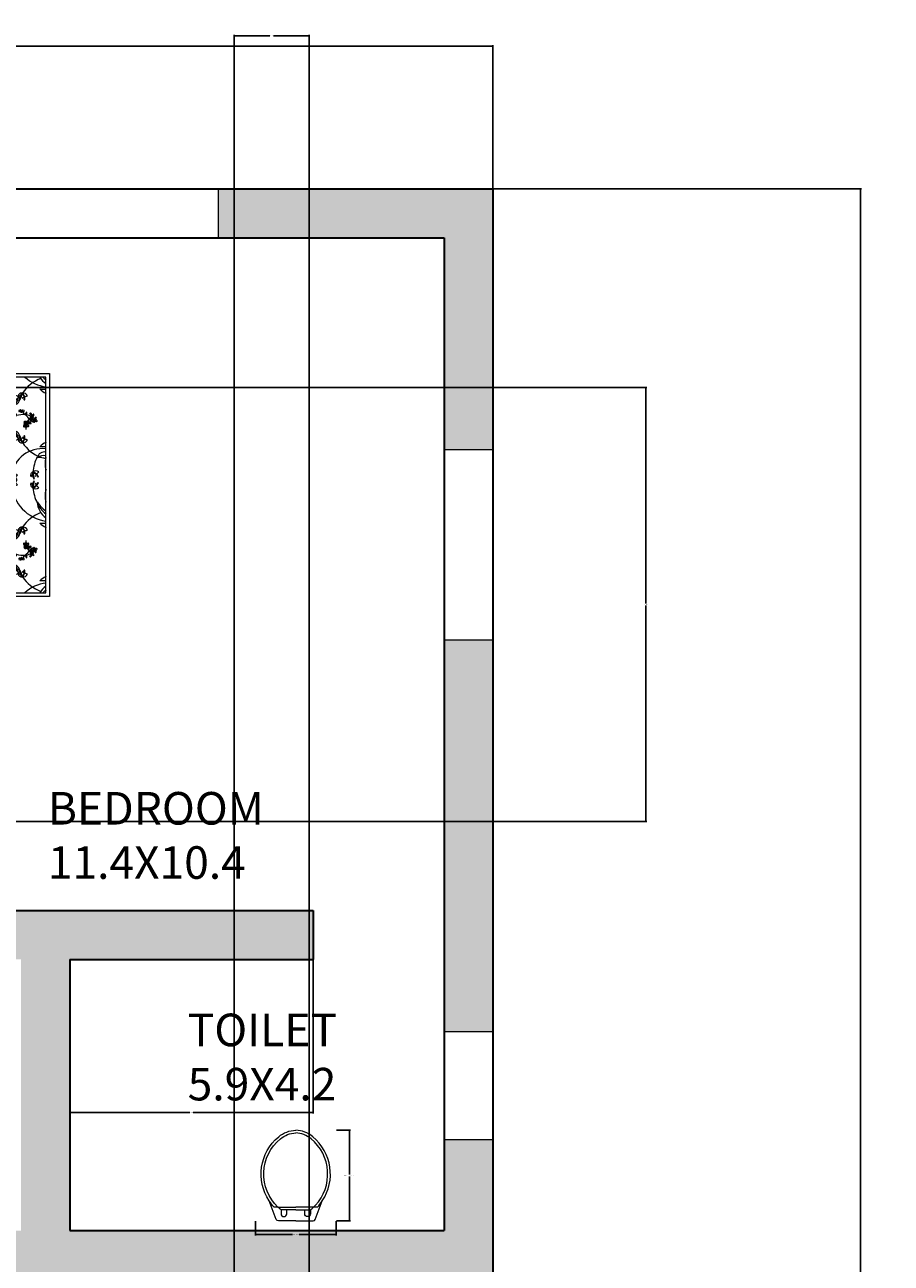
# Model space of a CAD drawing. Units: inches. Extents: x 8 to 486, y -516 to 97.
# Tile 5 of 5: x 326 to 486, y -185 to 43. Entities that reach past the tile are written whole.
import ezdxf

# ---------------------------------------------------------------- set-up
doc = ezdxf.new("R2010")
doc.units = ezdxf.units.IN
doc.header["$MEASUREMENT"] = 0
for name, color, linetype, lineweight in [('A-ANNO-DIMS', 2, 'Continuous', 18), ('A-AREA-IDEN', 7, 'Continuous', 18), ('A-FLOR-FIXT', 9, 'Continuous', 18), ('A-FURN', 8, 'Continuous', 18), ('A-GLAZ', 4, 'Continuous', 18), ('A-WALL', 7, 'Continuous', 35), ('A-WALL-PATT', 150, 'Continuous', 13)]:
    doc.layers.add(name, color=color, linetype=linetype, lineweight=lineweight)
doc.styles.get("Standard").update_dxf_attribs({"font": 'arial.ttf'})
doc.dimstyles.get("Standard").update_dxf_attribs({"dimtxt": 0.18, "dimasz": 0.18, "dimexe": 0.18, "dimexo": 0.0625, "dimgap": 0.09, "dimtad": 0, "dimtih": 1, "dimtoh": 1, "dimdec": 0, "dimzin": 0, "dimdsep": 46, "dimlunit": 3, "dimtxsty": 'Standard', "dimcen": 0.09, "dimadec": 0, "dimazin": 0, "dimtfac": 1, "dimtdec": 0, "dimtofl": 0, "dimtmove": 0, "dimatfit": 3, "dimfxl": 1, "dimtolj": 1, "dimtzin": 0, "dimarcsym": 0})

# ---------------------------------------------------------------- blocks, each defined once
blk = doc.blocks.new('*D1')
at = {"layer": 'A-ANNO-DIMS', "color": 0, "lineweight": -2, "transparency": 16777216}
for p, q in [((37.13, 12.8), (37.13, 39.25)), ((37.31, 39.07), (214.23, 39.07)), ((411.95, 39.07), (235.02, 39.07)), ((412.13, 12.8), (412.13, 39.25))]:
    blk.add_line(p, q, dxfattribs=at)
at = {"layer": 'A-ANNO-DIMS', "color": 0, "transparency": 16777216}
for points in [[(37.31, 39.1), (37.31, 39.04), (37.13, 39.07)], [(411.95, 39.1), (411.95, 39.04), (412.13, 39.07)]]:
    blk.add_solid(points, dxfattribs=at)
at = {"layer": 'Defpoints', "color": 0, "transparency": 16777216}
for p in [(412.13, 39.07), (37.13, 12.74), (412.13, 12.74)]:
    blk.add_point(p, dxfattribs=at)
at = {"layer": 'A-ANNO-DIMS', "color": 0, "transparency": 16777216, "insert": (224.63, 39.07), "char_height": 6, "attachment_point": 5}
blk.add_mtext('\\A1;31\'-3"', dxfattribs=at)
blk = doc.blocks.new('*D2')
at = {"layer": 'A-ANNO-DIMS', "color": 0, "lineweight": -2, "transparency": 16777216}
for p, q in [((412.19, 12.74), (480.06, 12.74)), ((479.88, 12.56), (479.88, -224.11)), ((479.88, -467.08), (479.88, -230.42)), ((412.19, -467.26), (480.06, -467.26))]:
    blk.add_line(p, q, dxfattribs=at)
at = {"layer": 'A-ANNO-DIMS', "color": 0, "transparency": 16777216}
for points in [[(479.85, 12.56), (479.91, 12.56), (479.88, 12.74)], [(479.85, -467.08), (479.91, -467.08), (479.88, -467.26)]]:
    blk.add_solid(points, dxfattribs=at)
at = {"layer": 'Defpoints', "color": 0, "transparency": 16777216}
for p in [(412.13, 12.74), (412.13, -467.26), (479.88, -467.26)]:
    blk.add_point(p, dxfattribs=at)
at = {"layer": 'A-ANNO-DIMS', "color": 0, "transparency": 16777216, "insert": (479.88, -227.26), "char_height": 6, "attachment_point": 5}
blk.add_mtext("\\A1;40'", dxfattribs=at)
blk = doc.blocks.new('BED-DOUBLE')
for p, q in [((0, 0), (0, 56.34)), ((4.7, 47.03), (4.7, 54.39)), ((8.38, 50.71), (1.01, 50.71)), ((27.62, 45.39), (27.62, 48.51)), ((27.62, 48.51), (47.92, 48.51)), ((47.92, 48.51), (47.92, 7.44)), ((28.27, 47.86), (28.27, 45.37)), ((47.26, 47.86), (28.27, 47.86)), ((47.26, 8.09), (47.26, 47.86)), ((0.72, 45.07), (0.72, 11.27)), ((8.9, 11.27), (8.9, 45.07)), ((11.24, 44.92), (11.53, 24.86)), ((11.82, 44.9), (12.11, 24.44)), ((13.6, 44.87), (13.68, 23.48)), ((14.18, 44.87), (14.26, 23.26)), ((31.13, 45.33), (31.13, 10.62)), ((31.84, 45.38), (31.84, 10.62)), ((41.55, 42.31), (40.91, 42.43)), ((37.37, 39.61), (37.37, 16.73)), ((41.55, 38.37), (40.91, 38.24)), ((8.9, 26.75), (13.2, 23.66)), ((10.58, 19.09), (8.9, 25.24)), ((13.2, 23.66), (16.51, 22.4)), ((16.51, 22.4), (17.99, 22.17)), ((17.99, 22.17), (17.54, 20.35)), ((12.06, 14.99), (10.58, 19.09)), ((16.85, 18.87), (16.51, 16.36)), ((17.54, 20.35), (16.85, 18.87)), ((16.51, 16.36), (16.28, 13.5)), ((41.55, 17.58), (40.91, 17.7)), ((13.66, 12.82), (12.06, 14.99)), ((16.05, 10.76), (13.66, 12.82)), ((16.28, 13.5), (16.51, 11.22)), ((41.55, 13.64), (40.91, 13.52)), ((0, 11.27), (15.46, 11.27)), ((4.7, 9.31), (4.7, 1.95)), ((16.51, 11.22), (16.05, 10.76)), ((27.62, 7.44), (27.62, 10.62)), ((28.27, 10.62), (28.27, 8.09)), ((47.92, 7.44), (27.62, 7.44)), ((28.27, 8.09), (47.26, 8.09)), ((8.38, 5.63), (1.01, 5.63))]:
    blk.add_line(p, q)
for points in [[(0, 45.07), (9.39, 45.07), (9.39, 56.34), (0, 56.34)], [(4.7, 50.71), (3.56, 50.05)], [(4.7, 50.71), (5.83, 50.05)], [(9.39, 11.27), (9.39, 0), (0, 0)], [(4.7, 5.63), (3.56, 6.29)], [(4.7, 5.63), (5.83, 6.29)]]:
    blk.add_lwpolyline(points)
for points in [[(30.69, 45.31, 0.056112), (33.79, 45.72, 0.095341), (36.78, 46.51)], [(1.4, 41.84, -0.074897), (5.08, 41.77, 0.472817)], [(5.29, 30.31, -0.14099), (1.54, 30.2, -0.235245)], [(5.29, 27.91, 0.14099), (1.54, 28.02, 0.235245)], [(1.4, 14.5, 0.074897), (5.08, 14.57, -0.472817)], [(21.21, 10.65, 0.001242), (31.9, 10.62, -0.127202), (37.23, 9.49)]]:
    blk.add_lwpolyline(points, format="xyb")
for centre, radius in [((4.7, 50.71), 2.63), ((4.7, 50.71), 1.31), ((43.59, 39.05), 0.143), ((45.1, 39.99), 0.143), ((43.59, 16.9), 0.143), ((45.1, 15.96), 0.143), ((4.7, 5.63), 2.63), ((4.7, 5.63), 1.31)]:
    blk.add_circle(centre, radius)
for centre, radius, start, end in [((37.06, 46.09), 0.514, 336.5219, 123.8264), ((92.17, 41.33), 54.82, 175.2402, 181.8035), ((48.98, 40.75), 7.36, 111.4092, 145.6135), ((48.25, 53.34), 7.36, 228.1144, 262.255), ((49.24, 49.64), 3.59, 209.8884, 236.5383), ((48.41, 47.64), 2.99, 221.0454, 247.4453), ((46.8, 55.83), 10.18, 266.3481, 272.5919), ((49.91, 50.93), 4.47, 223.5186, 233.6964), ((15.79, 146.07), 101.24, 266.1, 270.9282), ((19.47, 176.89), 132.06, 269.1145, 274.8735), ((41.34, 46.16), 4.26, 203.6453, 236.3329), ((39.29, 43.68), 0.951, 88.9462, 185.5144), ((39.99, 43.97), 1.69, 193.079, 274.7067), ((39.43, 43.29), 1.35, 7.1143, 95.0551), ((38.92, 42.76), 1.31, 338.5779, 68.4181), ((39.13, 43.52), 1.64, 305.9599, 357.6409), ((39.73, 45.27), 2.66, 288.2955, 328.7386), ((41.6, 43.6), 0.846, 19.1312, 189.736), ((41.34, 43.8), 1.06, 285.6955, 4.031), ((42.75, 42.66), 1.12, 128.4175, 173.8338), ((42.51, 43.77), 0.518, 126.7319, 206.0245), ((42.76, 44.31), 0.61, 76.272, 177.0484), ((41.84, 45.56), 1.26, 284.7031, 328.6173), ((43.59, 43.96), 1.16, 125.7657, 194.5347), ((37.88, 46.02), 5.15, 332.8176, 347.4827), ((43.08, 44.11), 0.816, 20.9613, 102.2885), ((43.52, 44.92), 0.614, 181.7131, 301.5367), ((41.51, 43.68), 1.86, 2.0648, 41.1598), ((42.63, 44.37), 0.602, 316.2238, 62.3173), ((42.98, 44.02), 0.048, 20.2667, 316.2271), ((43.23, 43.75), 0.0444, 52.0591, 168.5166), ((43.28, 43.74), 0.0914, 168.5166, 2.0648), ((-534.78, 10.78), 537.08, 2.8502, 3.3148), ((6.56, 34.66), 7.26, 78.2417, 114.8684), ((0.75, 39.83), 7.55, 348.9631, 14.8961), ((37.99, 41.7), 0.679, 196.6343, 225.5483), ((37.79, 44.6), 2.33, 259.249, 301.1782), ((37.99, 41.7), 0.679, 127.675, 162.5814), ((38.39, 42.79), 1.8, 240.8249, 340.7178), ((37.86, 41.99), 0.843, 246.1646, 318.4347), ((38.8, 40.44), 2.17, 85.2696, 124.215), ((38.72, 43.06), 1.62, 240.0851, 262.564), ((39.35, 40.67), 1.16, 74.8529, 138.4347), ((40.34, 43), 1.4, 196.8663, 330.0915), ((39.75, 42.12), 0.35, 254.8529, 12.6959), ((38.8, 40.44), 2.17, 53.6555, 57.2989), ((39.95, 45.3), 3.02, 273.4924, 303.7117), ((42.35, 41.59), 0.111, 125.0752, 284.7644), ((42.52, 41.63), 0.239, 127.3642, 168.4363), ((42.33, 41.83), 0.345, 277.4968, 341.2737), ((42.6, 41.67), 0.137, 88.1325, 178.8919), ((42.88, 41.52), 0.297, 136.3462, 189.6513), ((42.71, 41.49), 0.124, 189.6513, 312.3208), ((42.74, 41.83), 0.143, 183.2768, 356.7232), ((43.19, 41.58), 0.47, 164.2829, 186.9148), ((42.63, 41.57), 0.235, 312.3208, 40.2111), ((43.13, 41.84), 0.333, 201.6382, 274.947), ((42.69, 41.38), 0.436, 42.3896, 66.5724), ((47.08, 44.83), 5.35, 217.9541, 226.8459), ((43, 41.64), 0.237, 10.9597, 52.2379), ((43.15, 41.62), 0.11, 274.947, 37.5263), ((43.52, 40.99), 0.115, 112.5583, 214.2343), ((43.45, 41.2), 0.27, 265.7131, 351.6568), ((43.21, 41.35), 0.472, 297.3659, 329.344), ((42.85, 41.75), 0.905, 313.6929, 321.7899), ((43.85, 41.13), 0.296, 115.5379, 168.6744), ((42.85, 41.56), 0.89, 329.344, 349.7412), ((42.14, 41.35), 1.59, 352.8698, 1.6736), ((44.37, 41.03), 0.16, 33.0979, 123.1364), ((40.84, 38.77), 4.19, 31.1156, 34.8118), ((44.14, 40.76), 0.434, 2.3172, 70.5201), ((44.3, 40.81), 0.374, 352.6008, 57.1845), ((37.99, 38.97), 0.679, 134.4517, 156.7144), ((38.39, 37.89), 1.8, 19.2822, 119.1751), ((37.86, 38.68), 0.843, 41.5653, 113.8354), ((38.72, 37.62), 1.62, 97.436, 119.9149), ((39.35, 40.01), 1.16, 221.5653, 285.1471), ((40.34, 37.67), 1.4, 29.9085, 163.1337), ((39.75, 38.56), 0.35, 347.3041, 105.1471), ((40.21, 40.19), 0.177, 169.5864, 349.5616), ((40.28, 40.18), 0.109, 349.5616, 167.2949), ((43.11, 36.27), 4.67, 110.1059, 116.9968), ((41.55, 40.12), 0.296, 129.5056, 182.6421), ((40.7, 40.8), 0.89, 308.4388, 328.836), ((40.54, 41.53), 1.59, 296.5064, 305.3102), ((40.53, 40.71), 0.905, 336.3901, 344.4871), ((41.52, 40.48), 0.115, 83.9457, 185.6216), ((41.06, 40.58), 0.472, 328.836, 0.8141), ((41.3, 40.45), 0.27, 306.5232, 32.4668), ((41.62, 40.66), 0.115, 112.5583, 214.2343), ((41.55, 40.86), 0.27, 265.7131, 351.6568), ((41.31, 41.01), 0.472, 297.3659, 329.344), ((40.95, 41.42), 0.905, 313.6929, 321.7899), ((41.96, 40.8), 0.296, 115.5379, 168.6744), ((40.95, 41.22), 0.89, 329.344, 349.7412), ((43.11, 36.27), 4.67, 86.1723, 106.4158), ((40.24, 41.02), 1.59, 352.8698, 1.6736), ((43.2, 38.81), 0.111, 125.0752, 284.7644), ((43.37, 38.85), 0.239, 93.635, 168.4363), ((43.38, 40.15), 0.654, 253.6301, 325.4631), ((43.56, 39.24), 0.463, 82.0748, 142.6895), ((43.51, 39.88), 0.475, 228.342, 274.9894), ((43.34, 39.23), 0.141, 138.2946, 276.2474), ((43.39, 39.21), 0.196, 358.5719, 143.8954), ((43.18, 39.05), 0.345, 277.4968, 341.2737), ((43.46, 38.88), 0.137, 88.1325, 178.8919), ((43.51, 39.36), 0.197, 208.8493, 269.9355), ((43.34, 39.32), 0.226, 274.2123, 318.1587), ((43.23, 38.6), 2.34, 60.7959, 85.244), ((38.25, 35.23), 7.7, 37.8256, 47.7588), ((43.73, 38.74), 0.297, 136.3462, 189.6513), ((43.52, 39.8), 0.398, 273.8774, 357.1501), ((44.04, 38.79), 0.47, 164.2829, 186.9148), ((44.03, 39.09), 0.452, 121.9501, 165.2442), ((43.68, 40.08), 0.385, 262.0748, 308.2393), ((43.49, 38.79), 0.235, 312.3208, 40.2111), ((43.98, 39.06), 0.333, 201.6382, 274.947), ((43.71, 39.26), 0.095, 262.868, 7.094), ((43.54, 38.6), 0.436, 42.3896, 66.5724), ((43.7, 39.34), 0.283, 278.5614, 22.5914), ((43.86, 38.86), 0.237, 10.9597, 118.7804), ((46.34, 38.35), 2.81, 156.1523, 156.9499), ((43.86, 39.35), 0.142, 44.3732, 121.9501), ((44.3, 39.69), 0.398, 181.4625, 249.4747), ((46.34, 38.35), 2.81, 130.182, 149.456), ((44.23, 40), 0.385, 215.1128, 261.2773), ((44.54, 39.98), 0.654, 197.889, 269.722), ((44, 38.83), 0.11, 274.947, 37.5263), ((44.34, 39.76), 0.475, 248.3627, 295.0101), ((44.1, 39.16), 0.463, 20.6625, 81.2773), ((44.79, 39.95), 0.463, 139.3812, 199.9959), ((43.93, 40.29), 0.654, 310.9365, 22.7695), ((44.23, 40.25), 0.475, 285.6484, 332.2957), ((44.5, 40.65), 0.125, 135.7354, 318.1297), ((44.29, 40.86), 0.166, 315.7354, 31.1156), ((44.15, 40.5), 0.385, 319.3812, 5.5456), ((44.59, 40.65), 0.125, 68.2452, 250.6395), ((45.64, 38.3), 2.5, 111.7087, 116.2181), ((43.23, 38.6), 2.34, 47.5083, 55.9967), ((44.66, 40.89), 0.374, 252.8042, 349.6943), ((44.3, 40.22), 0.398, 331.1838, 51.6792), ((44.71, 39.75), 0.111, 125.0752, 284.7644), ((44.7, 40.92), 0.166, 248.2452, 323.6254), ((44.88, 39.79), 0.239, 93.635, 168.4363), ((44.55, 41.02), 0.434, 291.7087, 3.0299), ((44.85, 40.17), 0.141, 138.2946, 276.2474), ((44.69, 39.98), 0.345, 277.4968, 341.2737), ((44.9, 40.15), 0.196, 358.5719, 143.8954), ((41.46, 43.31), 4.19, 323.6254, 327.3216), ((44.97, 39.82), 0.137, 88.1325, 178.8919), ((45.02, 40.3), 0.197, 208.8493, 269.9355), ((44.85, 40.26), 0.226, 274.2123, 318.1587), ((45.24, 39.68), 0.297, 136.3462, 189.6513), ((45.07, 39.65), 0.124, 189.6513, 312.3208), ((44.89, 40.92), 0.16, 325.6077, 55.6462), ((45.55, 39.73), 0.47, 164.2829, 186.9148), ((45.54, 40.03), 0.452, 121.9501, 165.2442), ((45, 39.73), 0.235, 312.3208, 40.2111), ((45.5, 39.99), 0.333, 201.6382, 274.947), ((45.23, 40.2), 0.095, 262.868, 7.094), ((45.05, 39.54), 0.436, 42.3896, 66.5724), ((45.21, 40.28), 0.283, 278.5614, 22.5914), ((45.37, 39.79), 0.237, 10.9597, 118.7804), ((45.37, 40.29), 0.142, 44.3732, 121.9501), ((45.52, 39.77), 0.11, 274.947, 37.5263), ((11.26, 35.15), 9.9, 166.3427, 191.1841), ((1.3, 36.57), 7.17, 333.8761, 16.1746), ((37.99, 38.97), 0.679, 203.2856, 232.325), ((37.79, 36.08), 2.33, 58.8218, 100.2867), ((41.34, 34.52), 4.26, 123.6671, 158.5059), ((38.8, 40.23), 2.17, 235.785, 274.7304), ((39.99, 36.71), 1.69, 85.2933, 166.921), ((39.29, 37), 0.951, 174.4856, 271.0538), ((39.43, 37.39), 1.35, 264.9449, 352.8857), ((38.92, 37.92), 1.31, 291.5819, 21.4221), ((38.8, 40.23), 2.17, 302.7011, 306.3445), ((39.13, 37.16), 1.64, 2.3591, 54.0401), ((39.95, 35.38), 3.02, 56.2883, 86.5076), ((39.73, 35.4), 2.66, 31.2614, 71.7045), ((41.6, 37.08), 0.846, 170.264, 340.8688), ((42.75, 38.01), 1.12, 186.1662, 231.5825), ((41.34, 36.88), 1.06, 355.969, 74.3045), ((42.51, 36.91), 0.518, 153.9755, 233.2681), ((43.59, 36.72), 1.16, 165.4653, 234.2343), ((37.88, 34.66), 5.15, 12.5173, 27.1824), ((41.51, 37), 1.86, 318.8402, 357.9352), ((42.63, 36.3), 0.602, 297.6827, 43.7762), ((43.01, 36.67), 0.0796, 43.7762, 339.7183), ((43.28, 36.93), 0.0914, 357.9352, 191.4834), ((43.23, 36.92), 0.0444, 191.4834, 307.9409), ((43.56, 38.71), 0.124, 189.6513, 312.3208), ((46.34, 38.35), 2.81, 175.2415, 182.8929), ((46.55, 28.98), 5.69, 82.8636, 171.8197), ((42.76, 36.36), 0.61, 182.9516, 283.728), ((41.84, 35.12), 1.26, 31.3827, 75.2969), ((43.52, 35.75), 0.614, 58.4633, 178.2869), ((43.08, 36.57), 0.816, 257.7115, 339.0387), ((48.98, 39.93), 7.36, 214.3865, 248.5908), ((48.41, 33.04), 2.99, 112.5547, 138.9546), ((46.8, 24.84), 10.18, 87.4081, 93.6519), ((4.21, 30.97), 2.79, 153.3437, 196.1026), ((5.19, 31.35), 2.99, 335.0183, 18.5407), ((52.19, 29.78), 7.36, 152.5854, 175.5377), ((46.95, 32.74), 1.32, 76.3898, 169.0739), ((46.77, 31.74), 1.67, 72.8609, 131.9049), ((46.03, 29.72), 3.29, 68.117, 96.6195), ((51.13, 31.84), 4.05, 162.9798, 196.4569), ((7.17, 36.95), 6.9, 254.1707, 275.9871), ((41.09, 29.2), 0.61, 106.1963, 206.9726), ((39.66, 29.82), 1.26, 314.6273, 358.5415), ((41.98, 29.31), 1.16, 155.6899, 224.4589), ((41.47, 29.19), 0.816, 50.8855, 132.2127), ((41.44, 30.11), 0.614, 211.6373, 331.4609), ((40.94, 29.19), 0.602, 346.148, 92.2415), ((40.32, 28.03), 1.86, 31.989, 71.0841), ((36.01, 28.25), 5.15, 2.7418, 17.407), ((45.03, 29.77), 0.61, 106.1963, 206.9726), ((43.6, 30.38), 1.26, 314.6273, 358.5415), ((45.92, 29.87), 1.16, 155.6899, 224.4589), ((45.41, 29.75), 0.816, 50.8855, 132.2127), ((45.38, 30.68), 0.614, 211.6373, 331.4609), ((44.26, 28.59), 1.86, 31.989, 71.0841), ((39.95, 28.81), 5.15, 2.7418, 17.407), ((44.88, 29.75), 0.602, 346.148, 92.2415), ((53.22, 30.24), 5.98, 174.3643, 175.6213), ((57.31, 27.08), 10.69, 160.0972, 160.2783), ((11.47, 26.54), 10.04, 171.5249, 193.96), ((7.17, 21.26), 6.9, 84.0129, 105.8293), ((-1.76, 25.79), 9.94, 349.8617, 13.6238), ((41.09, 28.62), 0.61, 153.0274, 253.8037), ((39.66, 28), 1.26, 1.4585, 45.3727), ((41.98, 28.51), 1.16, 135.5411, 204.3101), ((36.01, 29.58), 5.15, 342.593, 357.2582), ((40.32, 29.8), 1.86, 288.9159, 328.011), ((40.94, 28.64), 0.602, 267.7585, 13.852), ((41.44, 27.71), 0.614, 28.5391, 148.3627), ((41.47, 28.64), 0.816, 227.7873, 309.1145), ((48.25, 28.61), 7.36, 184.4623, 262.255), ((41.42, 29.06), 0.048, 50.1909, 346.0209), ((41.45, 28.76), 0.0796, 13.852, 309.9245), ((41.82, 28.97), 0.0914, 198.4408, 31.989), ((41.77, 28.95), 0.0444, 81.9833, 198.4408), ((41.82, 28.86), 0.0914, 328.011, 161.5592), ((41.77, 28.87), 0.0444, 161.5592, 278.0167), ((45.03, 28.06), 0.61, 153.0274, 253.8037), ((43.6, 27.44), 1.26, 1.4585, 45.3727), ((45.92, 27.95), 1.16, 135.5411, 204.3101), ((39.95, 29.01), 5.15, 342.593, 357.2582), ((44.26, 29.23), 1.86, 288.9159, 328.011), ((44.88, 28.07), 0.602, 267.7585, 13.852), ((45.38, 27.15), 0.614, 28.5391, 148.3627), ((45.41, 28.08), 0.816, 227.7873, 309.1145), ((52.19, 28.04), 7.36, 184.4623, 207.4146), ((45.36, 29.62), 0.048, 50.1909, 346.0209), ((45.39, 28.2), 0.0796, 13.852, 309.9245), ((45.76, 29.53), 0.0914, 198.4408, 31.989), ((45.71, 29.52), 0.0444, 81.9833, 198.4408), ((45.76, 28.3), 0.0914, 328.011, 161.5592), ((45.71, 28.31), 0.0444, 161.5592, 278.0167), ((51.13, 25.99), 4.05, 163.5431, 197.0202), ((53.22, 27.59), 5.98, 184.3787, 185.6357), ((57.31, 30.74), 10.69, 199.7217, 199.9028), ((21.79, 22.22), 20.43, 172.2196, 189.497), ((-4.62, 20.49), 13.1, 348.0397, 19.2615), ((48.98, 16.02), 7.36, 111.4092, 145.6135), ((49.24, 24.92), 3.59, 181.272, 236.5383), ((51.16, 28.56), 6.65, 214.0123, 234.053), ((49.91, 26.21), 4.47, 197.8504, 233.6964), ((-3.3, 26.09), 21.85, 340.1194, 349.3383), ((18.04, 22.05), 0.136, 358.8623, 109.7536), ((46.8, 31.1), 10.18, 266.3481, 272.5919), ((48.41, 22.91), 2.99, 221.0454, 247.4453), ((-534.78, 45.56), 537.08, 356.6852, 357.1498), ((21.45, 16.81), 4.59, 156.2616, 191.3392), ((41.34, 21.43), 4.26, 201.4941, 236.3329), ((39.29, 18.95), 0.951, 88.9462, 185.5144), ((39.99, 19.24), 1.69, 193.079, 274.7067), ((39.43, 18.56), 1.35, 7.1143, 95.0551), ((38.92, 18.03), 1.31, 338.5779, 68.4181), ((39.13, 18.79), 1.64, 305.9599, 357.6409), ((39.73, 20.54), 2.66, 288.2955, 328.7386), ((41.6, 18.87), 0.846, 19.1312, 189.736), ((41.34, 19.07), 1.06, 285.6955, 4.031), ((42.75, 17.93), 1.12, 128.4175, 173.8338), ((42.51, 19.04), 0.518, 126.7319, 206.0245), ((42.76, 19.58), 0.61, 76.272, 177.0484), ((41.84, 20.83), 1.26, 284.7031, 328.6173), ((43.59, 19.23), 1.16, 125.7657, 194.5347), ((37.88, 21.29), 5.15, 332.8176, 347.4827), ((43.08, 19.38), 0.816, 20.9613, 102.2885), ((42.63, 19.64), 0.602, 316.2238, 62.3173), ((41.51, 18.95), 1.86, 2.0648, 41.1598), ((43.52, 20.19), 0.614, 181.7131, 301.5367), ((42.98, 19.29), 0.048, 20.2667, 316.2271), ((43.23, 19.02), 0.0444, 52.0591, 168.5166), ((43.28, 19.02), 0.0914, 168.5166, 2.0648), ((0.75, 16.51), 7.55, 345.1039, 11.0369), ((37.79, 19.87), 2.33, 259.7133, 301.1782), ((37.99, 16.98), 0.679, 127.675, 156.7144), ((96.02, 16.06), 58.65, 179.3433, 185.6887), ((37.99, 16.98), 0.679, 203.229, 225.5483), ((38.39, 18.06), 1.8, 240.8249, 340.7178), ((37.86, 17.26), 0.843, 246.1646, 318.4347), ((38.8, 15.72), 2.17, 85.2696, 124.215), ((38.72, 18.33), 1.62, 240.0851, 262.564), ((39.35, 15.94), 1.16, 74.8529, 138.4347), ((40.34, 18.28), 1.4, 196.8663, 330.0915), ((39.75, 17.39), 0.35, 254.8529, 12.6959), ((38.8, 15.72), 2.17, 53.6555, 57.2989), ((39.95, 20.57), 3.02, 273.4924, 303.7117), ((43.2, 17.14), 0.111, 75.2356, 234.9248), ((43.37, 17.09), 0.239, 191.5637, 266.365), ((43.51, 16.07), 0.475, 85.0106, 131.658), ((43.38, 15.8), 0.654, 34.5369, 106.3699), ((43.56, 16.71), 0.463, 217.3105, 277.9252), ((43.34, 16.72), 0.141, 83.7526, 221.7054), ((43.18, 16.9), 0.345, 18.7263, 82.5032), ((43.39, 16.74), 0.196, 216.1046, 1.4281), ((43.46, 17.06), 0.137, 181.1081, 271.8675), ((43.51, 16.58), 0.197, 90.0645, 151.1507), ((43.34, 16.63), 0.226, 41.8413, 85.7877), ((38.25, 20.72), 7.7, 312.2412, 322.1744), ((43.73, 17.21), 0.297, 170.3487, 223.6538), ((43.56, 17.24), 0.124, 47.6792, 170.3487), ((46.34, 17.59), 2.81, 177.1071, 184.7585), ((43.52, 16.15), 0.398, 2.8499, 86.1226), ((44.04, 17.15), 0.47, 173.0852, 195.7171), ((44.03, 16.86), 0.452, 194.7558, 238.0499), ((43.68, 15.87), 0.385, 51.7607, 97.9252), ((43.49, 17.16), 0.235, 319.7889, 47.6792), ((43.98, 16.89), 0.333, 85.053, 158.3618), ((43.71, 16.68), 0.095, 352.906, 97.132), ((43.54, 17.35), 0.436, 293.4276, 317.6104), ((43.86, 17.09), 0.237, 241.2196, 349.0403), ((43.7, 16.6), 0.283, 337.4086, 81.4386), ((46.34, 17.59), 2.81, 203.0501, 203.8477), ((43.86, 16.59), 0.142, 238.0499, 315.6268), ((44.3, 16.26), 0.398, 110.5253, 178.5375), ((44.54, 15.97), 0.654, 90.278, 162.111), ((44.23, 15.95), 0.385, 98.7227, 144.8872), ((46.34, 17.59), 2.81, 210.544, 229.818), ((44, 17.11), 0.11, 322.4737, 85.053), ((44.34, 16.19), 0.475, 64.9899, 111.6373), ((44.1, 16.78), 0.463, 278.7227, 339.3375), ((44.79, 15.99), 0.463, 160.0041, 220.6188), ((43.93, 15.66), 0.654, 337.2305, 49.0635), ((44.23, 15.7), 0.475, 27.7043, 74.3516), ((44.71, 16.2), 0.111, 75.2356, 234.9248), ((44.88, 16.16), 0.239, 191.5637, 266.365), ((44.69, 15.96), 0.345, 18.7263, 82.5032), ((44.97, 16.12), 0.137, 181.1081, 271.8675), ((45.07, 16.3), 0.124, 47.6792, 170.3487), ((45.24, 16.27), 0.297, 170.3487, 223.6538), ((45.55, 16.21), 0.47, 173.0852, 195.7171), ((45, 16.22), 0.235, 319.7889, 47.6792), ((45.5, 15.95), 0.333, 85.053, 158.3618), ((45.05, 16.41), 0.436, 293.4276, 317.6104), ((45.37, 16.15), 0.237, 241.2196, 349.0403), ((45.52, 16.18), 0.11, 322.4737, 85.053), ((6.56, 21.68), 7.26, 245.1316, 281.7583), ((-3.9, 11.73), 21.26, 357.4519, 11.3392), ((37.99, 14.24), 0.679, 134.4517, 153.558), ((37.99, 14.24), 0.679, 210.0293, 232.325), ((38.39, 13.16), 1.8, 19.2822, 119.1751), ((37.86, 13.96), 0.843, 41.5653, 113.8354), ((38.8, 15.5), 2.17, 235.785, 274.7304), ((38.72, 12.89), 1.62, 97.436, 119.9149), ((39.35, 15.28), 1.16, 221.5653, 285.1471), ((40.34, 12.94), 1.4, 29.9085, 163.1337), ((39.75, 13.83), 0.35, 347.3041, 105.1471), ((38.8, 15.5), 2.17, 302.7011, 306.3445), ((40.21, 15.76), 0.177, 10.4384, 190.4136), ((39.13, 12.43), 1.64, 2.3591, 54.0401), ((40.28, 15.77), 0.109, 192.7051, 10.4384), ((43.11, 19.68), 4.67, 243.0032, 249.8941), ((40.7, 15.15), 0.89, 31.164, 51.5612), ((41.55, 15.83), 0.296, 177.3579, 230.4944), ((40.54, 14.42), 1.59, 54.6898, 63.4936), ((40.53, 15.24), 0.905, 15.5129, 23.6099), ((41.52, 15.47), 0.115, 174.3784, 276.0543), ((41.3, 15.5), 0.27, 327.5332, 53.4768), ((41.06, 15.36), 0.472, 359.1859, 31.164), ((41.62, 15.29), 0.115, 145.7657, 247.4417), ((41.55, 15.09), 0.27, 8.3432, 94.2869), ((41.31, 14.94), 0.472, 30.656, 62.6341), ((40.95, 14.53), 0.905, 38.2101, 46.3071), ((41.96, 15.15), 0.296, 191.3256, 244.4621), ((40.95, 14.72), 0.89, 10.2588, 30.656), ((43.11, 19.68), 4.67, 253.5842, 273.8277), ((40.24, 14.93), 1.59, 358.3264, 7.1302), ((42.35, 14.36), 0.111, 75.2356, 234.9248), ((42.52, 14.31), 0.239, 191.5637, 232.6358), ((42.33, 14.12), 0.345, 18.7263, 82.5032), ((42.6, 14.28), 0.137, 181.1081, 271.8675), ((42.88, 14.43), 0.297, 170.3487, 223.6538), ((42.71, 14.46), 0.124, 47.6792, 170.3487), ((42.74, 14.11), 0.143, 3.2768, 176.7232), ((43.19, 14.37), 0.47, 173.0852, 195.7171), ((42.63, 14.37), 0.235, 319.7889, 47.6792), ((43.13, 14.11), 0.333, 85.053, 158.3618), ((42.69, 14.57), 0.436, 293.4276, 317.6104), ((47.08, 11.12), 5.35, 133.1541, 142.0459), ((43, 14.31), 0.237, 307.7621, 349.0403), ((43.15, 14.33), 0.11, 322.4737, 85.053), ((43.52, 14.96), 0.115, 145.7657, 247.4417), ((43.23, 17.35), 2.34, 274.756, 299.2041), ((43.45, 14.75), 0.27, 8.3432, 94.2869), ((43.21, 14.6), 0.472, 30.656, 62.6341), ((42.85, 14.2), 0.905, 38.2101, 46.3071), ((43.85, 14.81), 0.296, 191.3256, 244.4621), ((42.85, 14.39), 0.89, 10.2588, 30.656), ((42.14, 14.59), 1.59, 358.3264, 7.1302), ((44.14, 15.19), 0.434, 289.4799, 357.6828), ((40.84, 17.17), 4.19, 325.1882, 328.8844), ((44.37, 14.91), 0.16, 236.8636, 326.9021), ((44.5, 15.3), 0.125, 41.8703, 224.2646), ((44.29, 15.09), 0.166, 328.8844, 44.2646), ((44.15, 15.44), 0.385, 354.4544, 40.6188), ((44.59, 15.29), 0.125, 109.3605, 291.7548), ((44.3, 15.14), 0.374, 302.8155, 7.3992), ((45.64, 17.65), 2.5, 243.7819, 248.2913), ((43.23, 17.35), 2.34, 304.0033, 312.4917), ((44.3, 15.72), 0.398, 308.3208, 28.8162), ((44.66, 15.06), 0.374, 10.3057, 107.1958), ((44.7, 15.02), 0.166, 36.3746, 111.7548), ((44.85, 15.78), 0.141, 83.7526, 221.7054), ((44.55, 14.92), 0.434, 356.9701, 68.2913), ((44.9, 15.8), 0.196, 216.1046, 1.4281), ((41.46, 12.64), 4.19, 32.6784, 36.3746), ((45.02, 15.65), 0.197, 90.0645, 151.1507), ((44.85, 15.69), 0.226, 41.8413, 85.7877), ((44.89, 15.03), 0.16, 304.3538, 34.3923), ((45.54, 15.92), 0.452, 194.7558, 238.0499), ((45.23, 15.75), 0.095, 352.906, 97.132), ((45.21, 15.67), 0.283, 337.4086, 81.4386), ((45.37, 15.66), 0.142, 238.0499, 315.6268), ((37.79, 11.35), 2.33, 58.8218, 99.1554), ((41.34, 9.79), 4.26, 123.6671, 153.2997), ((39.99, 11.98), 1.69, 85.2933, 166.921), ((39.29, 12.27), 0.951, 174.4856, 271.0538), ((39.43, 12.66), 1.35, 264.9449, 352.8857), ((38.92, 13.19), 1.31, 291.5819, 21.4221), ((39.95, 10.65), 3.02, 56.2883, 86.5076), ((39.73, 10.68), 2.66, 31.2614, 71.7045), ((41.6, 12.35), 0.846, 170.264, 340.8688), ((41.34, 12.15), 1.06, 355.969, 74.3045), ((42.75, 13.29), 1.12, 186.1662, 231.5825), ((42.51, 12.18), 0.518, 153.9755, 233.2681), ((41.84, 10.39), 1.26, 31.3827, 75.2969), ((42.76, 11.64), 0.61, 182.9516, 283.728), ((43.59, 11.99), 1.16, 165.4653, 234.2343), ((37.88, 9.93), 5.15, 12.5173, 27.1824), ((41.51, 12.27), 1.86, 318.8402, 357.9352), ((42.63, 11.58), 0.602, 297.6827, 43.7762), ((43.52, 11.03), 0.614, 58.4633, 178.2869), ((43.08, 11.84), 0.816, 257.7115, 339.0387), ((43.01, 11.94), 0.0796, 43.7762, 339.7183), ((43.28, 12.2), 0.0914, 357.9352, 191.4834), ((43.23, 12.2), 0.0444, 191.4834, 307.9409), ((17.45, -40.9), 51.68, 85.8294, 91.553), ((37.19, 10.01), 0.52, 273.98, 27.3412), ((48.98, 15.2), 7.36, 214.3865, 248.5908), ((48.25, 2.61), 7.36, 97.745, 131.8856), ((49.24, 6.3), 3.59, 123.4617, 150.1116), ((48.41, 8.31), 2.99, 112.5547, 138.9546), ((46.8, 0.12), 10.18, 87.4081, 93.6519), ((49.91, 5.01), 4.47, 126.3036, 136.4814)]:
    blk.add_arc(centre, radius, start, end)
blk = doc.blocks.new('WC')
for p, q in [((3.1, 2.53), (2.4, 2.53)), ((3.1, 2.53), (6.39, 2.53)), ((9.68, 2.53), (6.39, 2.53)), ((10.38, 2.53), (9.68, 2.53))]:
    blk.add_line(p, q)
for points in [[(1.49, 3.68, -0.383919), (3.24, 15.51, -0.163732), (6.39, 16.72, -0.359733)], [(3.1, 2.53, -0.448546), (3.56, 15.13, -0.162618), (6.39, 16.22, -0.470877)], [(11.28, 3.68, 0.383919), (9.53, 15.51, 0.163732), (6.39, 16.72, 0.359733)], [(10.01, 2.87, 0.431639), (9.21, 15.13, 0.162618), (6.39, 16.22, 0.470877)], [(2.4, 2.53, -0.040937), (1.49, 3.68, -0.163732)], [(6.39, 0), (3.19, 0, -0.31031), (2.8, 0.27), (1.49, 3.68, -0.209071)], [(3.67, 2.03, -0.022712), (3.1, 2.53, -0.162618)], [(6.39, 0), (9.58, 0, 0.31031), (9.97, 0.27), (11.28, 3.68, 0.209071)], [(9.1, 2.03, 0.022712), (9.68, 2.53, 0.162618)], [(9.68, 2.53, 0.014165), (10.01, 2.87, 0.162618)], [(10.38, 2.53, 0.040937), (11.28, 3.68, 0.163732)], [(6.39, 2.03), (3.67, 2.03, -0.476108)], [(3.67, 2.03), (3.67, 1.33, 1), (4.74, 1.33), (4.74, 1.69)], [(6.39, 2.03), (9.1, 2.03, 0.022712)], [(9.1, 2.03), (9.1, 1.33, -1), (8.03, 1.33), (8.03, 1.69)]]:
    blk.add_lwpolyline(points, format="xyb")
for points in [[(4.74, 1.69), (4.74, 2.03)], [(8.03, 1.69), (8.03, 2.03)]]:
    blk.add_lwpolyline(points)
blk = doc.blocks.new('*D11')
at = {"layer": 'A-ANNO-DIMS', "color": 0, "lineweight": -2, "transparency": 16777216}
for p, q in [((383.28, -160.75), (385.9, -160.75)), ((385.72, -160.93), (385.72, -168.92)), ((385.72, -177.28), (385.72, -169.29)), ((383.28, -177.46), (385.9, -177.46))]:
    blk.add_line(p, q, dxfattribs=at)
at = {"layer": 'A-ANNO-DIMS', "color": 0, "transparency": 16777216}
for points in [[(385.69, -160.93), (385.75, -160.93), (385.72, -160.75)], [(385.69, -177.28), (385.75, -177.28), (385.72, -177.46)]]:
    blk.add_solid(points, dxfattribs=at)
at = {"layer": 'Defpoints', "color": 0, "transparency": 16777216}
for p in [(383.21, -160.75), (385.72, -160.75), (383.21, -177.46)]:
    blk.add_point(p, dxfattribs=at)
at = {"layer": 'A-ANNO-DIMS', "color": 0, "transparency": 16777216, "insert": (385.72, -169.1), "char_height": 0.18, "attachment_point": 5}
blk.add_mtext('\\A1;WC 1\'-4 1/2" TYP.', dxfattribs=at)
blk = doc.blocks.new('*D12')
at = {"layer": 'A-ANNO-DIMS', "color": 0, "lineweight": -2, "transparency": 16777216}
for p, q in [((368.36, -177.53), (368.36, -180.15)), ((383.21, -177.53), (383.21, -180.15)), ((368.54, -179.97), (375.16, -179.97)), ((383.03, -179.97), (376.42, -179.97))]:
    blk.add_line(p, q, dxfattribs=at)
at = {"layer": 'A-ANNO-DIMS', "color": 0, "transparency": 16777216}
for points in [[(368.54, -179.94), (368.54, -180), (368.36, -179.97)], [(383.03, -179.94), (383.03, -180), (383.21, -179.97)]]:
    blk.add_solid(points, dxfattribs=at)
at = {"layer": 'Defpoints', "color": 0, "transparency": 16777216}
for p in [(368.36, -177.46), (383.21, -177.46), (383.21, -179.97)]:
    blk.add_point(p, dxfattribs=at)
at = {"layer": 'A-ANNO-DIMS', "color": 0, "transparency": 16777216, "insert": (375.79, -179.97), "char_height": 0.18, "attachment_point": 5}
blk.add_mtext('\\A1;1\'-3" TYP.', dxfattribs=at)
blk = doc.blocks.new('*D31')
at = {"layer": 'A-ANNO-DIMS', "color": 0, "lineweight": -2, "transparency": 16777216}
for p, q in [((258.19, -23.87), (440.51, -23.87)), ((440.33, -24.05), (440.33, -63.69)), ((440.33, -103.69), (440.33, -64.05)), ((258.19, -103.87), (440.51, -103.87))]:
    blk.add_line(p, q, dxfattribs=at)
at = {"layer": 'A-ANNO-DIMS', "color": 0, "transparency": 16777216}
for points in [[(440.3, -24.05), (440.36, -24.05), (440.33, -23.87)], [(440.3, -103.69), (440.36, -103.69), (440.33, -103.87)]]:
    blk.add_solid(points, dxfattribs=at)
at = {"layer": 'Defpoints', "color": 0, "transparency": 16777216}
for p in [(258.13, -23.87), (258.13, -103.87), (440.33, -103.87)]:
    blk.add_point(p, dxfattribs=at)
at = {"layer": 'A-ANNO-DIMS', "color": 0, "transparency": 16777216, "insert": (440.33, -63.87), "char_height": 0.18, "attachment_point": 5}
blk.add_mtext('\\A1;6\'-8"', dxfattribs=at)
blk = doc.blocks.new('*D36')
at = {"layer": 'A-ANNO-DIMS', "color": 0, "lineweight": -2, "transparency": 16777216}
for p, q in [((364.45, -315.96), (364.45, 41.12)), ((378.23, -315.96), (378.23, 41.12)), ((364.63, 40.94), (371.02, 40.94)), ((378.05, 40.94), (371.66, 40.94))]:
    blk.add_line(p, q, dxfattribs=at)
at = {"layer": 'A-ANNO-DIMS', "color": 0, "transparency": 16777216}
for points in [[(364.63, 40.97), (364.63, 40.91), (364.45, 40.94)], [(378.05, 40.97), (378.05, 40.91), (378.23, 40.94)]]:
    blk.add_solid(points, dxfattribs=at)
at = {"layer": 'Defpoints', "color": 0, "transparency": 16777216}
for p in [(378.23, 40.94), (364.45, -316.02), (378.23, -316.02)]:
    blk.add_point(p, dxfattribs=at)
at = {"layer": 'A-ANNO-DIMS', "color": 0, "transparency": 16777216, "insert": (371.34, 40.94), "char_height": 0.18, "attachment_point": 5}
blk.add_mtext('\\A1;1\'-2"', dxfattribs=at)
blk = doc.blocks.new('*D43')
at = {"layer": 'A-ANNO-DIMS', "color": 0, "lineweight": -2, "transparency": 16777216}
for p, q in [((334.13, -129.33), (334.13, -157.64)), ((379.01, -129.33), (379.01, -157.64)), ((334.31, -157.46), (356.24, -157.46)), ((378.83, -157.46), (356.9, -157.46))]:
    blk.add_line(p, q, dxfattribs=at)
at = {"layer": 'A-ANNO-DIMS', "color": 0, "transparency": 16777216}
for points in [[(334.31, -157.43), (334.31, -157.49), (334.13, -157.46)], [(378.83, -157.43), (378.83, -157.49), (379.01, -157.46)]]:
    blk.add_solid(points, dxfattribs=at)
at = {"layer": 'Defpoints', "color": 0, "transparency": 16777216}
for p in [(334.13, -129.26), (379.01, -129.26), (334.13, -157.46)]:
    blk.add_point(p, dxfattribs=at)
at = {"layer": 'A-ANNO-DIMS', "color": 0, "transparency": 16777216, "insert": (356.57, -157.46), "char_height": 0.18, "attachment_point": 5}
blk.add_mtext('\\A1;3\'-9"', dxfattribs=at)

msp = doc.modelspace()

# ---------------------------------------------------------------- hatches: boundary and pattern name
at = {"layer": 'A-WALL-PATT'}
h = msp.add_hatch(color=256, dxfattribs=at)
h.dxf.hatch_style = 1
h.paths.add_polyline_path([(91.21, 12.74), (37.13, 12.74), (37.13, -29.65), (46.13, -29.65), (46.13, 3.74), (91.21, 3.74)])
h.paths.add_polyline_path([(211.13, 12.74), (137.85, 12.74), (137.85, 3.74), (182.13, 3.74), (182.13, -73.87), (191.13, -73.87), (191.13, 3.74), (211.13, 3.74)])
h.paths.add_polyline_path([(306.98, 12.74), (234.7, 12.74), (234.7, 3.74), (306.98, 3.74)])
h.paths.add_polyline_path([(267.13, 3.74), (258.13, 3.74), (258.13, -129.26), (267.13, -129.26)])
h.paths.add_polyline_path([(412.13, 12.74), (361.49, 12.74), (361.49, 3.74), (403.13, 3.74), (403.13, -35.28), (412.13, -35.28)])
h.paths.add_polyline_path([(379.01, -120.26), (297.29, -120.26), (297.29, -129.26), (325.13, -129.26), (325.13, -179.26), (218.14, -179.26), (218.14, -188.26), (325.13, -188.26), (325.13, -242.26), (297.29, -242.26), (297.29, -251.26), (379.01, -251.26), (379.01, -242.26), (334.13, -242.26), (334.13, -188.26), (403.13, -188.26), (403.13, -209.46), (412.13, -209.46), (412.13, -162.44), (403.13, -162.44), (403.13, -179.26), (334.13, -179.26), (334.13, -129.26), (379.01, -129.26)])
h.paths.add_polyline_path([(412.13, -70.38), (403.13, -70.38), (403.13, -142.55), (412.13, -142.55)])
h.paths.add_polyline_path([(412.13, -226.8), (403.13, -226.8), (403.13, -274.76), (412.13, -274.76)])
h.paths.add_polyline_path([(412.13, -317.95), (403.13, -317.95), (403.13, -361.26), (339.99, -361.26), (339.99, -370.26), (412.13, -370.26)])
h.paths.add_polyline_path([(412.13, -407.2), (403.13, -407.2), (403.13, -458.26), (373.42, -458.26), (373.42, -467.26), (412.13, -467.26)])
h.paths.add_polyline_path([(326.44, -458.26), (303.13, -458.26), (303.13, -283.74), (294.13, -283.74), (294.13, -416.26), (282.5, -416.26), (282.5, -425.26), (294.13, -425.26), (294.13, -467.26), (326.44, -467.26)])
h.paths.add_polyline_path([(246.84, -416.26), (233.38, -416.26), (233.38, -425.26), (246.84, -425.26)])
h.paths.add_polyline_path([(171.13, -307.26), (171.13, -191.26), (171.13, -182.26), (162.13, -182.26), (162.13, -191.26), (162.13, -307.26), (122.6, -307.26), (122.6, -316.26), (162.13, -316.26), (162.13, -425.26), (171.13, -425.26)])
h.paths.add_polyline_path([(84.39, -307.26), (46.13, -307.26), (46.13, -274.81), (37.13, -274.81), (37.13, -316.26), (84.39, -316.26)])
h.paths.add_polyline_path([(46.13, -191.26), (108.13, -191.26), (108.13, -182.26), (46.13, -182.26), (46.13, -172.25), (37.13, -172.25), (37.13, -224.84), (46.13, -224.84)])
h.paths.add_polyline_path([(191.13, -120.26), (46.13, -120.26), (46.13, -76.77), (37.13, -76.77), (37.13, -150.77), (46.13, -150.77), (46.13, -129.26), (99.13, -129.26), (99.13, -163.77), (108.13, -163.77), (108.13, -129.26), (191.13, -129.26)])

# ---------------------------------------------------------------- linework, layer by layer
at = {"layer": 'A-GLAZ'}
for p, q in [((361.49, 12.74), (361.49, 3.74)), ((403.13, -35.28), (412.13, -35.28)), ((403.13, -70.38), (412.13, -70.38)), ((403.13, -142.55), (412.13, -142.55)), ((403.13, -162.44), (412.13, -162.44))]:
    msp.add_line(p, q, dxfattribs=at)
at = {"layer": 'A-WALL'}
for p, q in [((37.13, 12.74), (412.13, 12.74)), ((412.13, 12.74), (412.13, -467.26)), ((191.13, 3.74), (403.13, 3.74)), ((403.13, 3.74), (403.13, -179.26)), ((297.29, -120.26), (379.01, -120.26)), ((379.01, -120.26), (379.01, -129.26)), ((334.13, -129.26), (334.13, -179.26)), ((334.13, -129.26), (379.01, -129.26)), ((334.13, -179.26), (403.13, -179.26))]:
    msp.add_line(p, q, dxfattribs=at)

# ---------------------------------------------------------------- block references
at = {"layer": 'A-FLOR-FIXT'}
msp.add_blockref('WC', (369.4, -177.46), dxfattribs=at)
at = {"layer": 'A-FURN'}
msp.add_blockref('BED-DOUBLE', (282.48, -69.79), dxfattribs=at)

# ---------------------------------------------------------------- texts
at = {"layer": 'A-AREA-IDEN', "char_height": 6, "attachment_point": 1}
for s, insert in [('BEDROOM\\P11.4X10.4', (330.08, -98.41)), ('TOILET\\P5.9X4.2', (355.86, -139.26))]:
    msp.add_mtext(s, dxfattribs=dict(at, insert=insert))

# ---------------------------------------------------------------- dimensions: what is measured, and where the dimension line sits
at = {"layer": 'A-ANNO-DIMS'}
for base, p1, p2, override, picture, middle in [((412.13, 39.07), (37.13, 12.74), (412.13, 12.74), {"dimtxt": 6, "dimclrd": 0, "dimclre": 0, "dimclrt": 0}, '*D1', (224.63, 39.07)), ((378.23, 40.94), (364.45, -316.02), (378.23, -316.02), {"dimdec": 1, "dimlfac": 1, "dimrnd": 0, "dimzin": 1, "dimdsep": 46, "dimlunit": 4, "dimfrac": 2}, '*D36', (371.34, 40.94))]:
    dim = msp.add_linear_dim(base=base, p1=p1, p2=p2, dimstyle='Standard', override=override, dxfattribs=at)
    dim.commit()
    dim.dimension.update_dxf_attribs({"geometry": picture, "text_midpoint": middle})
for base, p1, p2, angle, override, picture, middle in [((479.88, -467.26), (412.13, 12.74), (412.13, -467.26), 90, {"dimtxt": 6, "dimclrd": 0, "dimclre": 0, "dimclrt": 0}, '*D2', (479.88, -227.26)), ((440.33, -103.87), (258.13, -23.87), (258.13, -103.87), 90, {"dimdec": 1, "dimlfac": 1, "dimrnd": 0, "dimzin": 1, "dimdsep": 46, "dimlunit": 4, "dimfrac": 2}, '*D31', (440.33, -63.87)), ((334.13, -157.46), (379.01, -129.26), (334.13, -129.26), 180, {"dimdec": 1, "dimlfac": 1, "dimrnd": 0, "dimzin": 1, "dimdsep": 46, "dimlunit": 4, "dimfrac": 2}, '*D43', (356.57, -157.46))]:
    dim = msp.add_linear_dim(base=base, p1=p1, p2=p2, angle=angle, dimstyle='Standard', override=override, dxfattribs=at)
    dim.commit()
    dim.dimension.update_dxf_attribs({"geometry": picture, "text_midpoint": middle})
dim = msp.add_linear_dim(base=(385.72, -160.75), p1=(383.21, -177.46), p2=(383.21, -160.75), angle=90, text='WC <> TYP.', dimstyle='Standard', override={"dimdec": 1, "dimlfac": 1, "dimrnd": 0, "dimzin": 1, "dimdsep": 46, "dimlunit": 4, "dimfrac": 2}, dxfattribs=at)
dim.commit()
dim.dimension.update_dxf_attribs({"geometry": '*D11', "text_midpoint": (385.72, -169.1)})
dim = msp.add_linear_dim(base=(383.2128, -179.971), p1=(368.3603, -177.4634), p2=(383.2128, -177.4634), text='<> TYP.', dimstyle='Standard', override={"dimdec": 1, "dimlfac": 1, "dimrnd": 0, "dimzin": 1, "dimdsep": 46, "dimlunit": 4, "dimfrac": 2}, dxfattribs=at)
dim.commit()
dim.dimension.update_dxf_attribs({"geometry": '*D12', "text_midpoint": (375.7865, -179.971)})

doc.saveas('drawing.dxf')
